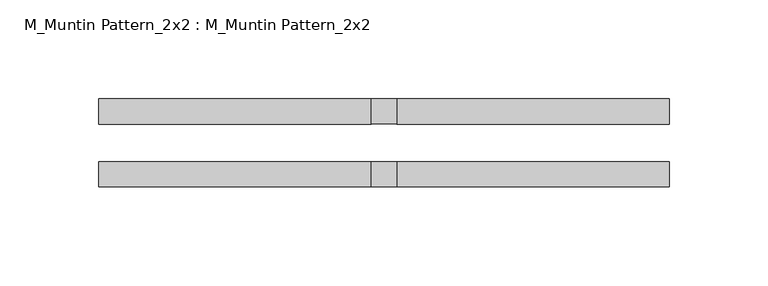
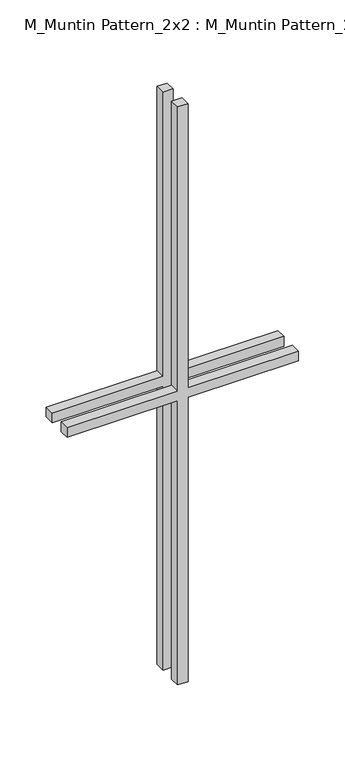
"""IFC4 building model written with IfcOpenShell, lengths in millimetres: proxy geometry, M_Muntin Pattern_2x2 : M_Muntin Pattern_2x2."""

from ifc_helpers import new_model, si_unit, frame, origin, place, context, project, spatial, polyline, outline, extrude, source, transform, mapped, element, save


def m_muntin_pattern_2x2_m_muntin_pattern_2x2_62480ac4(model_context):
    return source(origin(), model_context, "Body", "SweptSolid", [
        extrude(outline(polyline([(386.5, -6.35), (386.5, -144.2375), (373.8, -144.2375), (373.8, -6.35), (0.0, -6.35), (0.0, 6.35), (373.8, 6.35), (373.8, 144.2375), (386.5, 144.2375), (386.5, 6.35), (760.3, 6.35), (760.3, -6.35), (386.5, -6.35)])), frame((0.0, 9.525, 0.0), z_axis=(0.0, 1.0, 0.0), x_axis=(0.0, 0.0, 1.0)), (0.0, 0.0, 1.0), 12.7),
        extrude(outline(polyline([(386.5, -6.35), (386.5, -144.2375), (373.8, -144.2375), (373.8, -6.35), (0.0, -6.35), (0.0, 6.35), (373.8, 6.35), (373.8, 144.2375), (386.5, 144.2375), (386.5, 6.35), (760.3, 6.35), (760.3, -6.35), (386.5, -6.35)])), frame((0.0, -22.225, 0.0), z_axis=(0.0, 1.0, 0.0), x_axis=(0.0, 0.0, 1.0)), (0.0, 0.0, 1.0), 12.7),
    ])


if __name__ == "__main__":
    model = new_model("IFC4")
    model_context = context("Model", 3, world=origin())
    ifc_project = project(units=[si_unit("LENGTHUNIT", "METRE", prefix="MILLI")], contexts=[model_context])
    site = spatial("IfcSite", under=ifc_project)
    building = spatial("IfcBuilding", under=site)
    placement = place(None, origin())
    m_muntin_pattern_2x2_m_muntin_pattern_2x2_shape = m_muntin_pattern_2x2_m_muntin_pattern_2x2_62480ac4(model_context)
    element("IfcBuildingElementProxy", 1, Name="M_Muntin Pattern_2x2 : M_Muntin Pattern_2x2", ObjectType="M_Muntin Pattern_2x2 : M_Muntin Pattern_2x2", at=placement, inside=building, context=model_context, shape_type="MappedRepresentation", body=[
        mapped(m_muntin_pattern_2x2_m_muntin_pattern_2x2_shape, transform((0.0, 0.0, 0.0), x_axis=(1.0, 0.0, 0.0), y_axis=(0.0, 1.0, 0.0), z_axis=(0.0, 0.0, 1.0))),
    ])
    save(model, "model.ifc")

# Revit data of these elements
# Type "M_Muntin Pattern_2x2 : M_Muntin Pattern_2x2"
#   Width [instance default] = 1200 mm
#   Thickness = 12.7 mm
#   Height [instance default] = 1200 mm
#   Distance = 19.05 mm
#   Interior Material [instance default] = none
#   Exterior Material [instance default] = none
#   Default Elevation = 0
# Element 1 (IfcBuildingElementProxy, "M_Muntin Pattern_2x2 : M_Muntin Pattern_2x2")
#   Width = 288.475 mm
#   Height = 760.3 mm
#   Interior Material = Wood - Stained
#   Exterior Material = Clad - White
#   Materials on its faces: "Clad - White", "Wood - Stained"
# Materials
#   "Clad - White": class "Wood", colour RGB 242 242 238, transparency 0, Cost = 0
#   "Wood - Stained": class "Wood", colour RGB 224 178 126, transparency 0, Cost = 0
